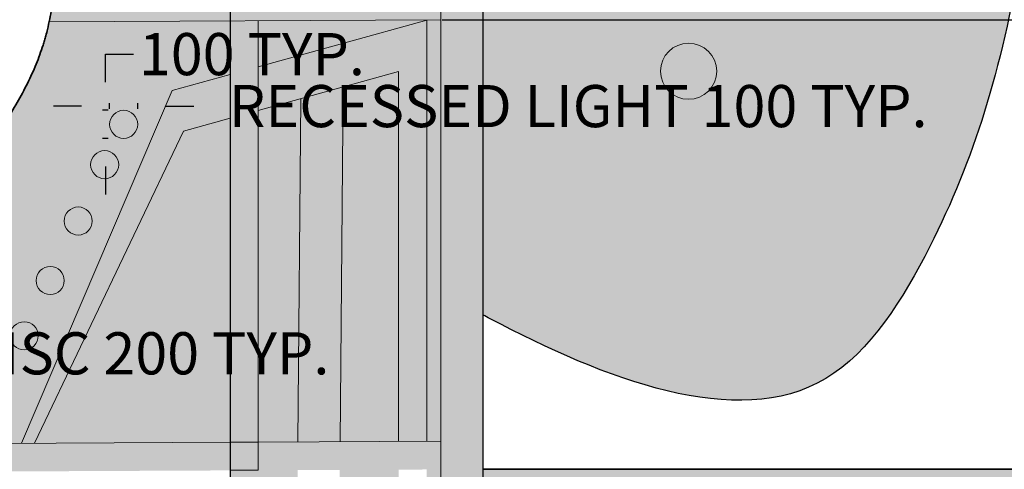
# Model space of a CAD drawing. Units: millimetres. Extents: x 11032 to 26788, y 3406 to 24505.
# Tile 69 of 78: x 21249 to 24753, y 11120 to 12721. Entities that reach past the tile are written whole.
import ezdxf

# ---------------------------------------------------------------- set-up
doc = ezdxf.new("R2010")
doc.units = ezdxf.units.MM
doc.header["$MEASUREMENT"] = 0
for name, color, linetype, lineweight in [('A-ANNO-DIMS', 2, 'Continuous', 18), ('A-GLAZ', 250, 'Continuous', 20), ('A-GLAZ-PATT', 9, 'Continuous', 13), ('A-ROOF', 7, 'Continuous', 30), ('A-WALL', 7, 'Continuous', 35), ('E-LITE', 7, 'Continuous', 18), ('E-LITE-PATT', 7, 'Continuous', 13)]:
    doc.layers.add(name, color=color, linetype=linetype, lineweight=lineweight)
for name, color, linetype, lineweight, true_color in [('A-GLAZ-FRAM-PATT', 250, 'Continuous', 13, 0x262627), ('A-ROOF-PATT', 9, 'Continuous', 13, 0xc7c8ca), ('A-WALL-CLAD-PATT', 9, 'Continuous', 13, 0xc7c8ca)]:
    doc.layers.add(name, color=color, linetype=linetype, lineweight=lineweight, true_color=true_color)
doc.styles.get("Standard").update_dxf_attribs({"font": 'arial.ttf'})
doc.dimstyles.get("Standard").update_dxf_attribs({"dimtxt": 150, "dimasz": 100, "dimexe": 10, "dimexo": 5, "dimgap": 5, "dimtad": 0, "dimtih": 1, "dimtoh": 1, "dimdec": 0, "dimzin": 0, "dimdsep": 46, "dimtxsty": 'Standard', "dimcen": 0.09, "dimadec": 0, "dimazin": 0, "dimtfac": 1, "dimtdec": 0, "dimtofl": 0, "dimtmove": 0, "dimatfit": 3, "dimfxl": 1, "dimtolj": 1, "dimtzin": 0, "dimarcsym": 0})

# ---------------------------------------------------------------- blocks, each defined once
blk = doc.blocks.new('RECESSED-LIGHT-100')
blk.add_circle((50, 50), 50)
blk = doc.blocks.new('RECESSED-LIGHT-200')
blk.add_circle((100, 100), 100)
blk = doc.blocks.new('*D20')
at = {"layer": 'A-ANNO-DIMS', "color": 0, "lineweight": -2, "transparency": 16777216}
for p, q in [((21468.9, 12413.4), (21368.9, 12413.4)), ((21568.9, 12403.4), (21568.9, 12423.4)), ((21668.9, 12403.4), (21668.9, 12423.4)), ((21768.9, 12413.4), (21868.9, 12413.4))]:
    blk.add_line(p, q, dxfattribs=at)
at = {"layer": 'A-ANNO-DIMS', "color": 0, "transparency": 16777216}
for points in [[(21468.9, 12430), (21468.9, 12396.7), (21568.9, 12413.4)], [(21768.9, 12430), (21768.9, 12396.7), (21668.9, 12413.4)]]:
    blk.add_solid(points, dxfattribs=at)
at = {"layer": 'Defpoints', "color": 0, "transparency": 16777216}
for p in [(21668.9, 12413.4), (21568.9, 12398.4), (21668.9, 12398.4)]:
    blk.add_point(p, dxfattribs=at)
at = {"layer": 'A-ANNO-DIMS', "color": 0, "transparency": 16777216, "insert": (23236.5, 12413.4), "char_height": 150, "attachment_point": 5}
blk.add_mtext('\\A1;RECESSED LIGHT 100 TYP.', dxfattribs=at)
blk = doc.blocks.new('*D21')
at = {"layer": 'A-ANNO-DIMS', "color": 0, "lineweight": -2, "transparency": 16777216}
for p, q in [((21553.9, 12498.4), (21553.9, 12598.4)), ((21553.9, 12598.4), (21653.9, 12598.4)), ((21563.9, 12398.4), (21543.9, 12398.4)), ((21563.9, 12298.4), (21543.9, 12298.4)), ((21553.9, 12198.4), (21553.9, 12098.4))]:
    blk.add_line(p, q, dxfattribs=at)
at = {"layer": 'A-ANNO-DIMS', "color": 0, "transparency": 16777216}
for points in [[(21537.2, 12498.4), (21570.6, 12498.4), (21553.9, 12398.4)], [(21537.2, 12198.4), (21570.6, 12198.4), (21553.9, 12298.4)]]:
    blk.add_solid(points, dxfattribs=at)
at = {"layer": 'Defpoints', "color": 0, "transparency": 16777216}
for p in [(21553.9, 12398.4), (21568.9, 12398.4), (21568.9, 12298.4)]:
    blk.add_point(p, dxfattribs=at)
at = {"layer": 'A-ANNO-DIMS', "color": 0, "transparency": 16777216, "insert": (22075.2, 12598.4), "char_height": 150, "attachment_point": 5}
blk.add_mtext('\\A1;100 TYP.', dxfattribs=at)
blk = doc.blocks.new('*D32')
at = {"layer": 'A-ANNO-DIMS', "color": 0, "lineweight": -2, "transparency": 16777216}
for p, q in [((19866, 11533.3), (19766, 11533.3)), ((19966, 11558.3), (19966, 11523.3)), ((20166, 11558.3), (20166, 11523.3)), ((20266, 11533.3), (20366, 11533.3))]:
    blk.add_line(p, q, dxfattribs=at)
at = {"layer": 'A-ANNO-DIMS', "color": 0, "transparency": 16777216}
for points in [[(19866, 11549.9), (19866, 11516.6), (19966, 11533.3)], [(20266, 11549.9), (20266, 11516.6), (20166, 11533.3)]]:
    blk.add_solid(points, dxfattribs=at)
at = {"layer": 'Defpoints', "color": 0, "transparency": 16777216}
for p in [(19966, 11563.3), (20166, 11563.3), (20166, 11533.3)]:
    blk.add_point(p, dxfattribs=at)
at = {"layer": 'A-ANNO-DIMS', "color": 0, "transparency": 16777216, "insert": (21400.3, 11533.3), "char_height": 150, "attachment_point": 5}
blk.add_mtext('\\A1;INLAY DISC 200 TYP.', dxfattribs=at)
blk = doc.blocks.new('*D36')
at = {"layer": 'A-ANNO-DIMS', "color": 0, "lineweight": -2, "transparency": 16777216}
for p, q in [((12301.3, 17115.9), (12301.3, 24416.9)), ((12401.3, 24406.9), (18569.2, 24406.9)), ((25297.4, 24406.9), (19129.5, 24406.9)), ((25397.4, 4466.4), (25397.4, 24416.9))]:
    blk.add_line(p, q, dxfattribs=at)
at = {"layer": 'A-ANNO-DIMS', "color": 0, "transparency": 16777216}
for points in [[(12401.3, 24423.5), (12401.3, 24390.2), (12301.3, 24406.9)], [(25297.4, 24423.5), (25297.4, 24390.2), (25397.4, 24406.9)]]:
    blk.add_solid(points, dxfattribs=at)
at = {"layer": 'Defpoints', "color": 0, "transparency": 16777216}
for p in [(25397.4, 24406.9), (12301.3, 17110.9), (25397.4, 4461.4)]:
    blk.add_point(p, dxfattribs=at)
at = {"layer": 'A-ANNO-DIMS', "color": 0, "transparency": 16777216, "insert": (18849.3, 24406.9), "char_height": 150, "attachment_point": 5}
blk.add_mtext('\\A1;13096', dxfattribs=at)
blk = doc.blocks.new('*D41')
at = {"layer": 'A-ANNO-DIMS', "color": 0, "lineweight": -2, "transparency": 16777216}
for p, q in [((22752.4, 12720.1), (26363.9, 12720.1)), ((26353.9, 12620.1), (26353.9, 12002)), ((26353.9, 11220.8), (26353.9, 11838.8)), ((25402.4, 11120.8), (26363.9, 11120.8))]:
    blk.add_line(p, q, dxfattribs=at)
at = {"layer": 'A-ANNO-DIMS', "color": 0, "transparency": 16777216}
for points in [[(26337.2, 12620.1), (26370.6, 12620.1), (26353.9, 12720.1)], [(26337.2, 11220.8), (26370.6, 11220.8), (26353.9, 11120.8)]]:
    blk.add_solid(points, dxfattribs=at)
at = {"layer": 'Defpoints', "color": 0, "transparency": 16777216}
for p in [(22747.4, 12720.1), (26353.9, 12720.1), (25397.4, 11120.8)]:
    blk.add_point(p, dxfattribs=at)
at = {"layer": 'A-ANNO-DIMS', "color": 0, "transparency": 16777216, "insert": (26353.9, 11920.4), "char_height": 150, "attachment_point": 5}
blk.add_mtext('\\A1;1599.3', dxfattribs=at)
blk = doc.blocks.new('*D42')
at = {"layer": 'A-ANNO-DIMS', "color": 0, "lineweight": -2, "transparency": 16777216}
for p, q in [((22752.4, 13320.1), (26363.9, 13320.1)), ((26353.9, 13220.1), (26353.9, 13101.7)), ((26353.9, 12820.1), (26353.9, 12938.5)), ((22752.4, 12720.1), (26363.9, 12720.1))]:
    blk.add_line(p, q, dxfattribs=at)
at = {"layer": 'A-ANNO-DIMS', "color": 0, "transparency": 16777216}
for points in [[(26337.2, 13220.1), (26370.6, 13220.1), (26353.9, 13320.1)], [(26337.2, 12820.1), (26370.6, 12820.1), (26353.9, 12720.1)]]:
    blk.add_solid(points, dxfattribs=at)
at = {"layer": 'Defpoints', "color": 0, "transparency": 16777216}
for p in [(22747.4, 13320.1), (26353.9, 13320.1), (22747.4, 12720.1)]:
    blk.add_point(p, dxfattribs=at)
at = {"layer": 'A-ANNO-DIMS', "color": 0, "transparency": 16777216, "insert": (26353.9, 13020.1), "char_height": 150, "attachment_point": 5}
blk.add_mtext('\\A1;600', dxfattribs=at)
blk = doc.blocks.new('*D51')
at = {"layer": 'A-ANNO-DIMS', "color": 0, "lineweight": -2, "transparency": 16777216}
for p, q in [((19697.4, 16000.7), (19697.4, 3494.9)), ((21997.4, 16011.6), (21997.4, 3494.9)), ((19797.4, 3504.9), (20617.4, 3504.9)), ((21897.4, 3504.9), (21077.4, 3504.9))]:
    blk.add_line(p, q, dxfattribs=at)
at = {"layer": 'A-ANNO-DIMS', "color": 0, "transparency": 16777216}
for points in [[(19797.4, 3521.6), (19797.4, 3488.2), (19697.4, 3504.9)], [(21897.4, 3521.6), (21897.4, 3488.2), (21997.4, 3504.9)]]:
    blk.add_solid(points, dxfattribs=at)
at = {"layer": 'Defpoints', "color": 0, "transparency": 16777216}
for p in [(21997.4, 16016.6), (19697.4, 16005.7), (21997.4, 3504.9)]:
    blk.add_point(p, dxfattribs=at)
at = {"layer": 'A-ANNO-DIMS', "color": 0, "transparency": 16777216, "insert": (20847.4, 3504.9), "char_height": 150, "attachment_point": 5}
blk.add_mtext('\\A1;2300', dxfattribs=at)
blk = doc.blocks.new('*D52')
at = {"layer": 'A-ANNO-DIMS', "color": 0, "lineweight": -2, "transparency": 16777216}
for p, q in [((22897.4, 16213.4), (22897.4, 3494.9)), ((21997.4, 16011.6), (21997.4, 3494.9)), ((22097.4, 3504.9), (22277, 3504.9)), ((22797.4, 3504.9), (22617.9, 3504.9))]:
    blk.add_line(p, q, dxfattribs=at)
at = {"layer": 'A-ANNO-DIMS', "color": 0, "transparency": 16777216}
for points in [[(22097.4, 3521.6), (22097.4, 3488.2), (21997.4, 3504.9)], [(22797.4, 3521.6), (22797.4, 3488.2), (22897.4, 3504.9)]]:
    blk.add_solid(points, dxfattribs=at)
at = {"layer": 'Defpoints', "color": 0, "transparency": 16777216}
for p in [(22897.4, 16218.4), (21997.4, 16016.6), (22897.4, 3504.9)]:
    blk.add_point(p, dxfattribs=at)
at = {"layer": 'A-ANNO-DIMS', "color": 0, "transparency": 16777216, "insert": (22447.4, 3504.9), "char_height": 150, "attachment_point": 5}
blk.add_mtext('\\A1;900', dxfattribs=at)
blk = doc.blocks.new('*D53')
at = {"layer": 'A-ANNO-DIMS', "color": 0, "lineweight": -2, "transparency": 16777216}
for p, q in [((22897.4, 11115.8), (22897.4, 3494.9)), ((25397.4, 11115.8), (25397.4, 3494.9)), ((22997.4, 3504.9), (23917.4, 3504.9)), ((25297.4, 3504.9), (24377.4, 3504.9))]:
    blk.add_line(p, q, dxfattribs=at)
at = {"layer": 'A-ANNO-DIMS', "color": 0, "transparency": 16777216}
for points in [[(22997.4, 3521.6), (22997.4, 3488.2), (22897.4, 3504.9)], [(25297.4, 3521.6), (25297.4, 3488.2), (25397.4, 3504.9)]]:
    blk.add_solid(points, dxfattribs=at)
at = {"layer": 'Defpoints', "color": 0, "transparency": 16777216}
for p in [(22897.4, 11120.8), (25397.4, 11120.8), (25397.4, 3504.9)]:
    blk.add_point(p, dxfattribs=at)
at = {"layer": 'A-ANNO-DIMS', "color": 0, "transparency": 16777216, "insert": (24147.4, 3504.9), "char_height": 150, "attachment_point": 5}
blk.add_mtext('\\A1;2500', dxfattribs=at)

msp = doc.modelspace()

# ---------------------------------------------------------------- hatches: boundary and pattern name
at = {"layer": 'A-GLAZ-FRAM-PATT'}
h = msp.add_hatch(color=256, dxfattribs=at)
h.paths.add_polyline_path([(22747.404, 16218.44), (22395.025, 16218.44), (18518.2, 16200.148), (18519.143, 16000.151), (22747.404, 16020.1)])
edge = h.paths.add_edge_path()
edge.add_line((22897.404, 16218.44), (22747.404, 16218.44))
edge.add_line((22747.404, 16218.44), (22747.404, 16020.1))
edge.add_line((22747.404, 16020.1), (22747.404, 9631.346))
edge.add_spline(control_points=[(22747.404, 9631.346), (22803.273, 9520.228), (22853.467, 9405.87), (22897.404, 9289.211)], knot_values=[2645.78092422, 2645.78092422, 2645.78092422, 2645.78092422, 3013.05623672, 3013.05623672, 3013.05623672, 3013.05623672], degree=3, periodic=0)
edge.add_line((22897.404, 9289.211), (22897.404, 16218.44))
h.paths.add_polyline_path([(22097.404, 16017.033), (21997.404, 16016.562), (21997.404, 13316.532), (22097.404, 13317.003)])
edge = h.paths.add_edge_path()
edge.add_line((19797.404, 16006.182), (19697.404, 16005.71))
edge.add_line((19697.404, 16005.71), (19697.404, 15155.703))
edge.add_line((19697.404, 15155.703), (19697.404, 12747.012))
edge.add_spline(control_points=[(19697.404, 12747.012), (19708.389, 12750.081), (19719.253, 12753.406), (19732.457, 12757.789), (19734.918, 12758.62), (19737.372, 12759.464)], knot_values=[1372.60477099, 1372.60477099, 1372.60477099, 1372.60477099, 1399.44343377, 1399.44343377, 1405.61279972, 1405.61279972, 1405.61279972, 1405.61279972], degree=3, periodic=0)
edge.add_spline(control_points=[(19737.372, 12759.464), (19750.245, 12763.891), (19762.932, 12768.657), (19778.9, 12775.14), (19782.354, 12776.572), (19785.794, 12778.028)], knot_values=[1405.61279972, 1405.61279972, 1405.61279972, 1405.61279972, 1437.96891336, 1437.96891336, 1446.94640473, 1446.94640473, 1446.94640473, 1446.94640473], degree=3, periodic=0)
edge.add_spline(control_points=[(19785.794, 12778.028), (19789.682, 12779.673), (19793.552, 12781.348), (19797.404, 12783.051)], knot_values=[1446.94640473, 1446.94640473, 1446.94640473, 1446.94640473, 1457.09545574, 1457.09545574, 1457.09545574, 1457.09545574], degree=3, periodic=0)
edge.add_line((19797.404, 12783.051), (19797.404, 15306.174))
edge.add_line((19797.404, 15306.174), (19797.404, 16006.182))
h = msp.add_hatch(color=256, dxfattribs=at)
h.paths.add_polyline_path([(22747.404, 16020.1), (22697.404, 16019.864), (22697.404, 15169.858), (22747.404, 15170.094)])
h.paths.add_polyline_path([(22747.404, 15070.092), (22697.404, 15069.857), (22697.404, 13319.834), (22747.404, 13320.07)])
edge = h.paths.add_edge_path()
edge.add_line((22747.404, 12795.064), (21365.955, 12788.546))
edge.add_spline(control_points=[(21365.955, 12788.546), (21365.556, 12785.216), (21365.14, 12781.894), (21364.707, 12778.582)], knot_values=[4871.89074498, 4871.89074498, 4871.89074498, 4871.89074498, 4881.51384723, 4881.51384723, 4881.51384723, 4881.51384723], degree=3, periodic=0)
edge.add_spline(control_points=[(21364.707, 12778.582), (21363.953, 12772.805), (21363.147, 12767.057), (21359.867, 12745.141), (21357.035, 12729.186), (21353.796, 12713.488)], knot_values=[4881.51384723, 4881.51384723, 4881.51384723, 4881.51384723, 4898.30109774, 4898.30109774, 4945.85686537, 4945.85686537, 4945.85686537, 4945.85686537], degree=3, periodic=0)
edge.add_line((21353.796, 12713.488), (22747.404, 12720.064))
edge.add_line((22747.404, 12720.064), (22747.404, 12795.064))
edge = h.paths.add_edge_path()
edge.add_line((22747.404, 13320.07), (22697.404, 13319.834))
edge.add_line((22697.404, 13319.834), (21312.567, 13313.3))
edge.add_spline(control_points=[(21312.567, 13313.3), (21312.567, 13313.3), (21312.567, 13313.3), (21312.567, 13313.3)], knot_values=[4405.86932069, 4405.86932069, 4405.86932069, 4405.86932069, 4405.86932536, 4405.86932536, 4405.86932536, 4405.86932536], degree=3, periodic=0)
edge.add_spline(control_points=[(21312.567, 13313.3), (21316.329, 13300.292), (21319.935, 13287.252), (21326.522, 13262.273), (21329.53, 13250.337), (21332.397, 13238.393)], knot_values=[4405.86932536, 4405.86932536, 4405.86932536, 4405.86932536, 4439.73791994, 4439.73791994, 4470.65028407, 4470.65028407, 4470.65028407, 4470.65028407], degree=3, periodic=0)
edge.add_line((21332.397, 13238.393), (22747.404, 13245.069))
edge.add_line((22747.404, 13245.069), (22747.404, 13320.07))
h.paths.add_polyline_path([(22747.404, 13245.069), (22697.404, 13244.833), (22697.404, 12794.828), (22747.404, 12795.064)])
h.paths.add_polyline_path([(22747.404, 12720.064), (22697.404, 12719.828), (22697.404, 11219.811), (22747.404, 11220.047)])
edge = h.paths.add_edge_path()
edge.add_line((22747.404, 11120.046), (22697.404, 11119.81))
edge.add_line((22697.404, 11119.81), (22697.404, 9727.135))
edge.add_spline(control_points=[(22697.404, 9727.135), (22714.538, 9695.493), (22731.209, 9663.555), (22747.404, 9631.346)], knot_values=[2539.32128955, 2539.32128955, 2539.32128955, 2539.32128955, 2645.78092422, 2645.78092422, 2645.78092422, 2645.78092422], degree=3, periodic=0)
edge.add_line((22747.404, 9631.346), (22747.404, 11120.046))
h = msp.add_hatch(color=256, dxfattribs=at)
h.paths.add_polyline_path([(21997.404, 12525.979), (21791.467, 12468.949), (21255.866, 11213.01), (21301.184, 11213.223), (21831.499, 12324.39), (21997.404, 12370.333)])
h.paths.add_polyline_path([(22697.404, 12719.828), (22097.404, 12716.997), (22097.404, 12553.671)])
h = msp.add_hatch(color=256, dxfattribs=at)
h.paths.add_polyline_path([(22097.404, 12716.997), (21997.404, 12716.525), (21997.404, 11216.508), (22097.404, 11216.508)])
h.paths.add_polyline_path([(22747.404, 11220.047), (22097.404, 11216.98), (22097.404, 11116.979), (22747.404, 11120.046)])
edge = h.paths.add_edge_path()
edge.add_line((22097.404, 11116.979), (21997.404, 11116.979))
edge.add_line((21997.404, 11116.979), (21997.404, 10579.29))
edge.add_spline(control_points=[(21997.404, 10579.29), (22031.89, 10555.567), (22065.161, 10529.697), (22097.404, 10502.28)], knot_values=[1427.45738773, 1427.45738773, 1427.45738773, 1427.45738773, 1555.90366196, 1555.90366196, 1555.90366196, 1555.90366196], degree=3, periodic=0)
edge.add_line((22097.404, 10502.28), (22097.404, 11116.979))
h.paths.add_polyline_path([(22097.404, 11216.508), (21997.404, 11216.508), (21997.404, 11116.979), (22097.404, 11116.979)])
h = msp.add_hatch(color=256, dxfattribs=at)
edge = h.paths.add_edge_path()
edge.add_line((21997.404, 11116.507), (21997.404, 11216.508))
edge.add_line((21997.404, 11216.508), (20604.964, 11209.938))
edge.add_spline(control_points=[(20604.964, 11209.938), (20607.134, 11206.535), (20609.342, 11203.201), (20617.481, 11191.329), (20623.597, 11183.201), (20636.089, 11167.852), (20642.464, 11160.629), (20655.347, 11147.002), (20661.856, 11140.596), (20674.924, 11128.498), (20681.484, 11122.806), (20690.98, 11115.01), (20693.915, 11112.662), (20696.848, 11110.371)], knot_values=[6471.16279551, 6471.16279551, 6471.16279551, 6471.16279551, 6478.49642841, 6478.49642841, 6497.82694928, 6497.82694928, 6517.15747016, 6517.15747016, 6536.48799103, 6536.48799103, 6555.81851191, 6555.81851191, 6564.46246221, 6564.46246221, 6564.46246221, 6564.46246221], degree=3, periodic=0)
edge.add_line((20696.848, 11110.371), (21997.404, 11116.507))
at = {"layer": 'A-GLAZ-PATT'}
h = msp.add_hatch(color=256, dxfattribs=at)
h.set_gradient(color1=(147, 149, 152), color2=(254, 234, 185), name='INVCURVED')
h.paths.add_polyline_path([(22597.404, 11219.339), (22697.404, 11219.811), (22697.404, 12719.828), (22097.404, 12553.671), (22097.404, 12398.026), (22597.404, 12536.49)])
h.paths.add_polyline_path([(22399.472, 12481.677), (22249.118, 12440.04), (22238.879, 11217.648), (22388.89, 11218.355)])
h = msp.add_hatch(color=256, dxfattribs=at)
h.set_gradient(color1=(254, 204, 102), color2=(248, 246, 176), name='HEMISPHERICAL')
edge = h.paths.add_edge_path()
edge.add_spline(control_points=[(21353.796, 12713.488), (21351.921, 12704.4), (21349.909, 12695.398), (21345.944, 12678.95), (21344.029, 12671.478), (21341.252, 12661.256), (21340.473, 12658.452), (21338.881, 12652.839), (21338.068, 12650.032), (21335.58, 12641.609), (21333.854, 12635.993), (21328.479, 12619.14), (21324.632, 12607.899), (21312.219, 12573.877), (21302.855, 12551.077), (21282.165, 12505.474), (21270.839, 12482.672), (21246.416, 12437.152), (21233.319, 12414.435), (21205.588, 12369.182), (21190.953, 12346.647), (21160.407, 12301.852), (21144.496, 12279.592), (21111.679, 12235.428), (21094.773, 12213.524), (21055.718, 12164.423), (21033.359, 12137.352), (20988.115, 12083.954), (20965.231, 12057.628), (20919.516, 12005.731), (20896.686, 11980.16), (20857.367, 11936.124), (20840.745, 11917.509), (20808.035, 11880.563), (20791.947, 11862.233), (20763.475, 11829.178), (20750.967, 11814.43), (20726.5, 11784.882), (20714.539, 11770.084), (20693.385, 11742.981), (20684.087, 11730.721), (20665.941, 11705.856), (20657.092, 11693.252), (20641.315, 11669.592), (20634.312, 11658.625), (20620.703, 11636.087), (20614.097, 11624.517), (20601.376, 11600.52), (20595.259, 11588.093), (20585.03, 11565.079), (20580.781, 11554.73), (20572.815, 11533.181), (20569.097, 11521.98), (20562.398, 11498.577), (20559.418, 11486.373), (20555.045, 11463.74), (20553.448, 11453.531), (20551.046, 11432.459), (20550.243, 11421.596), (20549.62, 11399.291), (20549.802, 11387.848), (20551.33, 11364.54), (20552.678, 11352.676), (20556.671, 11328.775), (20559.317, 11316.74), (20565.954, 11292.813), (20569.944, 11280.922), (20579.202, 11257.616), (20584.469, 11246.202), (20592.114, 11231.712), (20593.991, 11228.293), (20597.158, 11222.745), (20598.418, 11220.59), (20600.975, 11216.322), (20602.269, 11214.214), (20604.037, 11211.397), (20604.5, 11210.666), (20604.964, 11209.938)], knot_values=[4945.85686537, 4945.85686537, 4945.85686537, 4945.85686537, 4973.3893459, 4973.3893459, 4996.66899489, 4996.66899489, 5005.51338613, 5005.51338613, 5014.35777737, 5014.35777737, 5032.04655985, 5032.04655985, 5067.42412481, 5067.42412481, 5139.05868364, 5139.05868364, 5210.69324248, 5210.69324248, 5282.32780131, 5282.32780131, 5353.96236015, 5353.96236015, 5425.59691898, 5425.59691898, 5497.23147782, 5497.23147782, 5587.7210555, 5587.7210555, 5678.21063318, 5678.21063318, 5768.70021086, 5768.70021086, 5836.11850381, 5836.11850381, 5903.53679676, 5903.53679676, 5958.13178915, 5958.13178915, 6012.72678154, 6012.72678154, 6057.24703228, 6057.24703228, 6101.76728303, 6101.76728303, 6138.92040589, 6138.92040589, 6176.07352875, 6176.07352875, 6213.2266516, 6213.2266516, 6241.78247951, 6241.78247951, 6270.33830742, 6270.33830742, 6298.89413533, 6298.89413533, 6321.01839771, 6321.01839771, 6343.1426601, 6343.1426601, 6365.26692248, 6365.26692248, 6387.39118486, 6387.39118486, 6409.51544725, 6409.51544725, 6431.63970963, 6431.63970963, 6453.76397201, 6453.76397201, 6460.69362746, 6460.69362746, 6465.1443277, 6465.1443277, 6469.59502793, 6469.59502793, 6471.16279551, 6471.16279551, 6471.16279551, 6471.16279551], degree=3, periodic=0)
edge.add_line((20604.964, 11209.938), (21255.866, 11213.01))
edge.add_line((21255.866, 11213.01), (21791.467, 12468.949))
edge.add_line((21791.467, 12468.949), (21997.404, 12525.979))
edge.add_line((21997.404, 12525.979), (21997.404, 12716.525))
edge.add_line((21997.404, 12716.525), (21353.796, 12713.488))
h.paths.add_polyline_path([(21407.506, 11792.395, -1), (21307.506, 11792.395, -1)], flags=16)
h.paths.add_polyline_path([(21315.053, 11595.746, -1), (21215.053, 11595.746, -1)], flags=16)
h.paths.add_polyline_path([(21407.11, 12004.255, -1), (21507.11, 12004.255, -1)], flags=16)
h.paths.add_polyline_path([(21220.849, 11395.371, -1), (21120.849, 11395.371, -1)], flags=16)
h.paths.add_polyline_path([(21501.367, 12204.741, -1), (21601.367, 12204.741, -1)], flags=16)
h.paths.add_polyline_path([(21568.897, 12348.379, -1), (21668.897, 12348.379, -1)], flags=16)
h = msp.add_hatch(color=256, dxfattribs=at)
h.set_gradient(color1=(254, 234, 185), color2=(247, 242, 129), name='SPHERICAL')
h.paths.add_polyline_path([(22097.404, 11216.98), (22238.879, 11217.648), (22249.118, 12440.04), (22097.404, 12398.026)])
h.paths.add_polyline_path([(22597.404, 12536.49), (22399.472, 12481.677), (22388.89, 11218.355), (22597.404, 11219.339)])
edge = h.paths.add_edge_path()
edge.add_spline(control_points=[(22380.418, 10206.878), (22458.962, 10109.885), (22531.093, 10007.052), (22597.404, 9899.872)], knot_values=[1967.32460229, 1967.32460229, 1967.32460229, 1967.32460229, 2342.00276579, 2342.00276579, 2342.00276579, 2342.00276579], degree=3, periodic=0)
edge.add_line((22597.404, 9899.872), (22597.404, 10880.68))
edge.add_line((22597.404, 10880.68), (22385.926, 10864.474))
edge.add_line((22385.926, 10864.474), (22380.418, 10206.878))
edge = h.paths.add_edge_path()
edge.add_spline(control_points=[(22097.404, 10502.28), (22137.084, 10468.539), (22182.031, 10425.998), (22225.292, 10381.762), (22231.821, 10375.007)], knot_values=[1555.90366196, 1555.90366196, 1555.90366196, 1555.90366196, 1713.9810301, 1742.27732176, 1742.27732176, 1742.27732176, 1742.27732176], degree=3, periodic=0)
edge.add_line((22231.821, 10375.007), (22238.042, 11117.642))
edge.add_line((22238.042, 11117.642), (22097.404, 11116.979))
edge.add_line((22097.404, 11116.979), (22097.404, 10502.28))
h.paths.add_polyline_path([(22597.404, 10980.973), (22597.404, 11119.338), (22388.053, 11118.35), (22386.767, 10964.831)])
h = msp.add_hatch(color=256, dxfattribs=at)
h.set_gradient(color1=(254, 204, 102), color2=(248, 246, 176), name='HEMISPHERICAL')
h.paths.add_polyline_path([(21997.404, 12370.333), (21831.499, 12324.39), (21301.184, 11213.223), (21997.404, 11216.508)])
at = {"layer": 'A-ROOF-PATT'}
h = msp.add_hatch(color=256, dxfattribs=at)
h.set_gradient(color1=(254, 234, 185), color2=(254, 204, 102), name='HEMISPHERICAL')
edge = h.paths.add_edge_path()
edge.add_spline(control_points=[(22897.404, 11669.966), (22905.925, 11665.421), (23315.936, 11448.075), (24040.798, 11159.928), (24591.756, 12047.169), (24823.737, 12810.982), (24947.403, 13888.961), (24865.187, 14241.353)], knot_values=[3287.74811127, 3287.74811127, 3287.74811127, 3287.74811127, 3313.95061448, 4543.69878516, 5160.49832431, 6201.61230094, 7164.26935092, 7164.26935092, 7164.26935092, 7164.26935092], degree=3, periodic=0)
edge.add_spline(control_points=[(24865.187, 14241.353), (24864.423, 14242.575), (24766.311, 14398.016), (24602.876, 14465.087), (24430.499, 14490.269)], knot_values=[2462.20964139, 2462.20964139, 2462.20964139, 2462.20964139, 2466.8266732, 3052.28296943, 3052.28296943, 3052.28296943, 3052.28296943], degree=3, periodic=0)
edge.add_spline(control_points=[(24430.499, 14490.269), (24425.883, 14491.82), (24421.191, 14493.323), (24402.038, 14499.174), (24386.985, 14503.129), (24351.089, 14511.181), (24329.855, 14514.969), (24285.944, 14521.074), (24263.27, 14523.392), (24216.998, 14526.696), (24193.401, 14527.682), (24156.534, 14528.34), (24143.408, 14528.404), (24117.112, 14528.234), (24103.938, 14528.001), (24070.613, 14527.088), (24050.758, 14526.245), (24021.415, 14524.553), (24011.706, 14523.918), (23966.994, 14520.648), (23932.846, 14517.154), (23866.075, 14508.38), (23833.453, 14503.099), (23769.399, 14490.798), (23737.967, 14483.778), (23675.954, 14468.02), (23645.373, 14459.282), (23584.735, 14440.092), (23554.677, 14429.638), (23494.779, 14407.002), (23464.938, 14394.819), (23420.13, 14375.236), (23405.186, 14368.49), (23382.735, 14358.043), (23375.245, 14354.506), (23363.999, 14349.118), (23360.248, 14347.308), (23354.645, 14344.586), (23352.794, 14343.684), (23350.017, 14342.326), (23349.099, 14341.876), (23346.705, 14340.7), (23345.24, 14339.978), (23338.743, 14336.765), (23333.903, 14334.336), (23322.952, 14328.714), (23316.906, 14325.517), (23304.544, 14318.72), (23298.224, 14315.118), (23284.755, 14307.106), (23277.606, 14302.694), (23262.032, 14292.682), (23253.61, 14287.081), (23235.154, 14274.351), (23225.122, 14267.224), (23200.911, 14249.486), (23186.304, 14238.46), (23150.266, 14210.435), (23128.041, 14192.649), (23080.227, 14153.32), (23055.083, 14132.223), (23027.357, 14108.523)], knot_values=[765.02120011, 765.02120011, 765.02120011, 765.02120011, 788.26421035, 788.26421035, 858.47024111, 858.47024111, 949.55129088, 949.55129088, 1040.63234064, 1040.63234064, 1131.71339041, 1131.71339041, 1181.69353236, 1181.69353236, 1231.67367431, 1231.67367431, 1308.31901537, 1308.31901537, 1346.64168591, 1346.64168591, 1486.09404767, 1486.09404767, 1625.54640943, 1625.54640943, 1764.99877119, 1764.99877119, 1904.45113295, 1904.45113295, 2043.90349471, 2043.90349471, 2183.35585648, 2183.35585648, 2253.08203736, 2253.08203736, 2287.9451278, 2287.9451278, 2305.37667302, 2305.37667302, 2313.97014819, 2313.97014819, 2318.26688578, 2318.26688578, 2325.26983634, 2325.26983634, 2349.68341829, 2349.68341829, 2381.60377634, 2381.60377634, 2413.52413439, 2413.52413439, 2445.44449243, 2445.44449243, 2477.36485048, 2477.36485048, 2509.28520853, 2509.28520853, 2547.80727814, 2547.80727814, 2595.07704725, 2595.07704725, 2638.35089074, 2638.35089074, 2638.35089074, 2638.35089074], degree=3, periodic=0)
edge.add_spline(control_points=[(23027.357, 14108.523), (23027.349, 14108.516), (23027.342, 14108.51), (23027.334, 14108.504), (22984.024, 14071.482), (22940.714, 14034.46), (22897.404, 13997.439)], knot_values=[697.41436256, 697.41436256, 697.41436256, 697.41436256, 697.4261083, 697.4261083, 697.4261083, 765.02120011, 765.02120011, 765.02120011, 765.02120011], degree=3, periodic=0)
edge.add_line((22897.404, 13997.439), (22897.404, 11669.966))
h.paths.add_polyline_path([(23729.349, 12537.488, -1), (23529.349, 12537.488, -1)], flags=16)
h.paths.add_polyline_path([(23963.611, 13699.89, -1), (24163.611, 13699.89, -1)], flags=16)
at = {"layer": 'A-WALL-CLAD-PATT'}
h = msp.add_hatch(color=256, dxfattribs=at)
edge = h.paths.add_edge_path()
edge.add_spline(control_points=[(24865.187, 14241.353), (24844.683, 14329.238), (24708.481, 14689.762), (23980.011, 14777.842), (23439.65, 14624.598), (23111.535, 14443.589), (22897.404, 14260.55)], knot_values=[765.02120011, 765.02120011, 765.02120011, 765.02120011, 1005.10337375, 1880.54593672, 2963.32805357, 3287.74811127, 3287.74811127, 3287.74811127, 3287.74811127], degree=3, periodic=0)
edge.add_line((22897.404, 14260.55), (22897.404, 13997.439))
edge.add_spline(control_points=[(22897.404, 13997.439), (22940.714, 14034.46), (22984.024, 14071.482), (23027.334, 14108.504), (23027.342, 14108.51), (23027.349, 14108.516), (23027.357, 14108.523)], knot_values=[697.41436256, 697.41436256, 697.41436256, 697.41436256, 765.00945437, 765.00945437, 765.00945437, 765.02120011, 765.02120011, 765.02120011, 765.02120011], degree=3, periodic=0)
edge.add_spline(control_points=[(23027.357, 14108.523), (23055.083, 14132.223), (23080.227, 14153.32), (23128.041, 14192.649), (23150.266, 14210.435), (23186.304, 14238.46), (23200.911, 14249.486), (23225.122, 14267.224), (23235.154, 14274.351), (23253.61, 14287.081), (23262.032, 14292.682), (23277.606, 14302.694), (23284.755, 14307.106), (23298.224, 14315.118), (23304.544, 14318.72), (23316.906, 14325.517), (23322.952, 14328.714), (23333.903, 14334.336), (23338.743, 14336.765), (23345.24, 14339.978), (23346.705, 14340.7), (23349.099, 14341.876), (23350.017, 14342.326), (23352.794, 14343.684), (23354.645, 14344.586), (23360.248, 14347.308), (23363.999, 14349.118), (23375.245, 14354.506), (23382.735, 14358.043), (23405.186, 14368.49), (23420.13, 14375.236), (23464.938, 14394.819), (23494.779, 14407.002), (23554.677, 14429.638), (23584.735, 14440.092), (23645.373, 14459.282), (23675.954, 14468.02), (23737.967, 14483.778), (23769.399, 14490.798), (23833.453, 14503.099), (23866.075, 14508.38), (23932.846, 14517.154), (23966.994, 14520.648), (24011.706, 14523.918), (24021.415, 14524.553), (24050.758, 14526.245), (24070.613, 14527.088), (24103.938, 14528.001), (24117.112, 14528.234), (24143.408, 14528.404), (24156.534, 14528.34), (24193.401, 14527.682), (24216.998, 14526.696), (24263.27, 14523.392), (24285.944, 14521.074), (24329.855, 14514.969), (24351.089, 14511.181), (24386.985, 14503.129), (24402.038, 14499.174), (24421.191, 14493.323), (24425.883, 14491.82), (24430.499, 14490.269)], knot_values=[765.02120011, 765.02120011, 765.02120011, 765.02120011, 808.29504361, 808.29504361, 855.56481272, 855.56481272, 894.08688233, 894.08688233, 926.00724037, 926.00724037, 957.92759842, 957.92759842, 989.84795647, 989.84795647, 1021.76831451, 1021.76831451, 1053.68867256, 1053.68867256, 1078.10225451, 1078.10225451, 1085.10520508, 1085.10520508, 1089.40194266, 1089.40194266, 1097.99541784, 1097.99541784, 1115.42696306, 1115.42696306, 1150.2900535, 1150.2900535, 1220.01623438, 1220.01623438, 1359.46859614, 1359.46859614, 1498.9209579, 1498.9209579, 1638.37331966, 1638.37331966, 1777.82568142, 1777.82568142, 1917.27804319, 1917.27804319, 2056.73040495, 2056.73040495, 2095.05307548, 2095.05307548, 2171.69841654, 2171.69841654, 2221.67855849, 2221.67855849, 2271.65870045, 2271.65870045, 2362.73975021, 2362.73975021, 2453.82079998, 2453.82079998, 2544.90184974, 2544.90184974, 2615.10788051, 2615.10788051, 2638.35089074, 2638.35089074, 2638.35089074, 2638.35089074], degree=3, periodic=0)
edge.add_spline(control_points=[(24430.499, 14490.269), (24602.876, 14465.087), (24766.311, 14398.016), (24864.423, 14242.575), (24865.187, 14241.353)], knot_values=[2462.20964139, 2462.20964139, 2462.20964139, 2462.20964139, 3047.66593763, 3052.28296943, 3052.28296943, 3052.28296943, 3052.28296943], degree=3, periodic=0)
h.paths.add_polyline_path([(25397.404, 11120.753), (22897.404, 11120.753), (22897.404, 10520.753), (25197.404, 10520.753), (25197.404, 9359.601), (25397.404, 9359.601)])
at = {"layer": 'E-LITE-PATT'}
h = msp.add_hatch(color=256, dxfattribs=at)
h.paths.add_polyline_path([(23729.349, 12537.488, 1), (23529.349, 12537.488, 1)])
h.paths.add_polyline_path([(24163.611, 13699.89, 1), (23963.611, 13699.89, 1)])
h.paths.add_polyline_path([(18790.086, 14298.34, 1), (18890.086, 14298.34, 1)])
h.paths.add_polyline_path([(19537.524, 14550.125, 1), (19437.524, 14550.125, 1)])
h.paths.add_polyline_path([(20194.664, 14380.821, 1), (20344.664, 14380.821, 1)])
h.paths.add_polyline_path([(20018.772, 14780.204, 1), (19868.772, 14780.204, 1)])
h.paths.add_polyline_path([(20594.425, 14224.541, 1), (20744.425, 14224.541, 1)])
h.paths.add_polyline_path([(21232.101, 14202.835, 1), (21332.101, 14202.835, 1)])
h.paths.add_polyline_path([(20854.127, 14602.218, 1), (20754.127, 14602.218, 1)])
h.paths.add_polyline_path([(21492.875, 14667.335, 1), (21392.875, 14667.335, 1)])
h.paths.add_polyline_path([(21005.138, 14988.578, 1), (20855.138, 14988.578, 1)])
h = msp.add_hatch(color=256, dxfattribs=at)
h.paths.add_polyline_path([(21120.849, 11395.371, 1), (21220.849, 11395.371, 1)])
h.paths.add_polyline_path([(21215.053, 11595.746, 1), (21315.053, 11595.746, 1)])
h.paths.add_polyline_path([(21407.506, 11792.395, 1), (21307.506, 11792.395, 1)])
h.paths.add_polyline_path([(21507.11, 12004.255, 1), (21407.11, 12004.255, 1)])
h.paths.add_polyline_path([(21501.367, 12204.741, 1), (21601.367, 12204.741, 1)])
h.paths.add_polyline_path([(21668.897, 12348.379, 1), (21568.897, 12348.379, 1)])
h.paths.add_polyline_path([(23729.349, 12537.488, 1), (23529.349, 12537.488, 1)])
h.paths.add_polyline_path([(23963.611, 13699.89, 1), (24163.611, 13699.89, 1)])
h.paths.add_polyline_path([(21492.875, 14667.335, 1), (21392.875, 14667.335, 1)])
h.paths.add_polyline_path([(21332.101, 14202.835, 1), (21232.101, 14202.835, 1)])
h.paths.add_polyline_path([(20744.425, 14224.541, 1), (20594.425, 14224.541, 1)])
h.paths.add_polyline_path([(20854.127, 14602.218, 1), (20754.127, 14602.218, 1)])
h.paths.add_polyline_path([(20947.253, 15061.599), (20912.335, 15061.434, 0.34563694), (20855.138, 14988.578, 1), (21005.138, 14988.578, 0.34827999)])
h = msp.add_hatch(color=256, dxfattribs=at)
h.paths.add_polyline_path([(23529.349, 12537.488, 1), (23729.349, 12537.488, 1)])
h.paths.add_polyline_path([(24163.611, 13699.89, 1), (23963.611, 13699.89, 1)])

# ---------------------------------------------------------------- linework, layer by layer
at = {"layer": 'A-GLAZ'}
for p, q in [((22747.404, 16218.44), (22747.404, 9631.346)), ((22897.404, 16218.44), (22897.404, 9289.211)), ((22747.404, 12720.064), (21353.796, 12713.488)), ((22697.404, 12719.828), (22097.404, 12553.671)), ((22697.404, 12719.828), (22697.404, 11219.811)), ((21997.404, 12716.525), (21997.404, 11216.508)), ((22097.404, 12716.997), (22097.404, 11216.98)), ((21997.404, 12525.979), (21791.467, 12468.949)), ((22597.404, 12536.49), (22097.404, 12398.026)), ((22597.404, 12536.49), (22597.404, 11219.811)), ((22399.472, 12481.677), (22388.89, 11218.355)), ((21791.467, 12468.949), (21255.866, 11213.01)), ((22249.118, 12440.04), (22238.879, 11217.648)), ((21997.404, 12370.333), (21831.499, 12324.39)), ((21831.499, 12324.39), (21301.184, 11213.223)), ((21997.404, 11216.508), (20604.964, 11209.938)), ((22747.404, 11220.047), (22097.404, 11216.98))]:
    msp.add_line(p, q, dxfattribs=at)
msp.add_lwpolyline([(21997.404, 11216.508), (22097.404, 11216.508), (22097.404, 11116.979), (21997.404, 11116.979)], close=True, dxfattribs=at)
at = {"layer": 'A-ROOF'}
msp.add_open_spline([(22897.404, 14260.55), (23111.535, 14443.589), (23439.65, 14624.598), (23980.011, 14777.842), (25027.484, 14651.191), (24844.989, 12880.959), (24591.756, 12047.169), (24040.798, 11159.928), (23315.936, 11448.075), (22905.925, 11665.421), (22897.404, 11669.966)], degree=3, knots=[765.02120011, 765.02120011, 765.02120011, 765.02120011, 1089.44125781, 2172.22337467, 3047.66593763, 4250.40516126, 5291.51913789, 5908.31867703, 7138.06684772, 7164.26935092, 7164.26935092, 7164.26935092, 7164.26935092], dxfattribs=at)
at = {"layer": 'A-WALL'}
msp.add_line((22897.404, 11120.753), (25397.404, 11120.753), dxfattribs=at)
msp.add_open_spline([(20781.73, 14097.965), (20784.285, 14097.292), (20787.436, 14096.331), (20794.831, 14093.655), (20799.074, 14091.941), (20808.517, 14087.64), (20813.716, 14085.055), (20824.925, 14078.948), (20830.934, 14075.426), (20843.621, 14067.418), (20850.299, 14062.932), (20864.197, 14052.997), (20871.416, 14047.547), (20889.597, 14033.059), (20900.79, 14023.505), (20923.774, 14002.511), (20935.566, 13991.072), (20959.505, 13966.429), (20971.653, 13953.226), (20996.104, 13925.188), (21008.407, 13910.354), (21032.993, 13879.192), (21045.278, 13862.864), (21075.715, 13820.438), (21093.762, 13793.504), (21129.039, 13737.067), (21146.269, 13707.566), (21179.532, 13646.451), (21195.565, 13614.838), (21226.093, 13549.956), (21240.587, 13516.686), (21267.729, 13448.943), (21280.375, 13414.47), (21303.538, 13344.776), (21314.054, 13309.556), (21332.704, 13238.828), (21340.837, 13203.321), (21354.5, 13132.481), (21360.029, 13097.149), (21368.306, 13027.119), (21371.052, 12992.421), (21373.63, 12924.101), (21373.462, 12890.481), (21370.13, 12824.718), (21366.968, 12792.577), (21358.463, 12735.763), (21353.621, 12710.793), (21345.944, 12678.95), (21344.029, 12671.478), (21341.252, 12661.256), (21340.473, 12658.452), (21338.881, 12652.839), (21338.068, 12650.032), (21335.58, 12641.609), (21333.854, 12635.993), (21328.479, 12619.14), (21324.632, 12607.899), (21312.219, 12573.877), (21302.855, 12551.077), (21282.165, 12505.474), (21270.839, 12482.672), (21246.416, 12437.152), (21233.319, 12414.435), (21205.588, 12369.182), (21190.953, 12346.647), (21160.407, 12301.852), (21144.496, 12279.592), (21111.679, 12235.428), (21094.773, 12213.524), (21055.718, 12164.423), (21033.359, 12137.352), (20988.115, 12083.954), (20965.231, 12057.628), (20919.516, 12005.731), (20896.686, 11980.16), (20857.367, 11936.124), (20840.745, 11917.509), (20808.035, 11880.563), (20791.947, 11862.233), (20763.475, 11829.178), (20750.967, 11814.43), (20726.5, 11784.882), (20714.539, 11770.084), (20693.385, 11742.981), (20684.087, 11730.721), (20665.941, 11705.856), (20657.092, 11693.252), (20641.315, 11669.592), (20634.312, 11658.625), (20620.703, 11636.087), (20614.097, 11624.517), (20601.376, 11600.52), (20595.259, 11588.093), (20585.03, 11565.079), (20580.781, 11554.73), (20572.815, 11533.181), (20569.097, 11521.98), (20562.398, 11498.577), (20559.418, 11486.373), (20555.045, 11463.74), (20553.448, 11453.531), (20551.046, 11432.459), (20550.243, 11421.596), (20549.62, 11399.291), (20549.802, 11387.848), (20551.33, 11364.54), (20552.678, 11352.676), (20556.671, 11328.775), (20559.317, 11316.74), (20565.954, 11292.813), (20569.944, 11280.922), (20579.202, 11257.616), (20584.469, 11246.202), (20592.114, 11231.712), (20593.991, 11228.293), (20597.158, 11222.745), (20598.418, 11220.59), (20600.975, 11216.322), (20602.269, 11214.214), (20606.192, 11207.964), (20608.863, 11203.899), (20617.481, 11191.329), (20623.597, 11183.201), (20636.089, 11167.852), (20642.464, 11160.629), (20655.347, 11147.002), (20661.856, 11140.596), (20674.924, 11128.498), (20681.484, 11122.806), (20694.608, 11112.032), (20701.171, 11106.95), (20714.277, 11097.303), (20720.82, 11092.738), (20737.095, 11081.899), (20746.81, 11075.891), (20766.189, 11064.614), (20775.854, 11059.347), (20795.171, 11049.382), (20804.823, 11044.686), (20824.152, 11035.736), (20833.829, 11031.484), (20853.244, 11023.327), (20862.982, 11019.423), (20887.017, 11010.17), (20901.366, 11004.975), (20930.315, 10995.005), (20944.916, 10990.23), (20967.117, 10983.27), (20974.61, 10980.971), (20982.141, 10978.705), (20982.141, 10978.705), (20982.141, 10978.705), (20982.141, 10978.705), (21260.768, 10894.876), (21539.396, 10811.046), (21803.195, 10686.28), (21811.686, 10678.824), (21810.573, 10681.187), (21811.406, 10681.686), (21870.06, 10660.606), (21925.845, 10628.283), (21978.958, 10591.693)], degree=3, knots=[3328.11564031, 3328.11564031, 3328.11564031, 3328.11564031, 3370.54654151, 3370.54654151, 3412.97744272, 3412.97744272, 3455.40834392, 3455.40834392, 3497.83924512, 3497.83924512, 3540.27014632, 3540.27014632, 3582.70104752, 3582.70104752, 3644.05325934, 3644.05325934, 3705.40547115, 3705.40547115, 3766.75768296, 3766.75768296, 3828.10989477, 3828.10989477, 3889.46210658, 3889.46210658, 3981.17474214, 3981.17474214, 4072.8873777, 4072.8873777, 4164.60001326, 4164.60001326, 4256.31264882, 4256.31264882, 4348.02528438, 4348.02528438, 4439.73791994, 4439.73791994, 4531.4505555, 4531.4505555, 4623.16319106, 4623.16319106, 4714.87582662, 4714.87582662, 4806.58846218, 4806.58846218, 4898.30109774, 4898.30109774, 4973.3893459, 4973.3893459, 4996.66899489, 4996.66899489, 5005.51338613, 5005.51338613, 5014.35777737, 5014.35777737, 5032.04655985, 5032.04655985, 5067.42412481, 5067.42412481, 5139.05868364, 5139.05868364, 5210.69324248, 5210.69324248, 5282.32780131, 5282.32780131, 5353.96236015, 5353.96236015, 5425.59691898, 5425.59691898, 5497.23147782, 5497.23147782, 5587.7210555, 5587.7210555, 5678.21063318, 5678.21063318, 5768.70021086, 5768.70021086, 5836.11850381, 5836.11850381, 5903.53679676, 5903.53679676, 5958.13178915, 5958.13178915, 6012.72678154, 6012.72678154, 6057.24703228, 6057.24703228, 6101.76728303, 6101.76728303, 6138.92040589, 6138.92040589, 6176.07352875, 6176.07352875, 6213.2266516, 6213.2266516, 6241.78247951, 6241.78247951, 6270.33830742, 6270.33830742, 6298.89413533, 6298.89413533, 6321.01839771, 6321.01839771, 6343.1426601, 6343.1426601, 6365.26692248, 6365.26692248, 6387.39118486, 6387.39118486, 6409.51544725, 6409.51544725, 6431.63970963, 6431.63970963, 6453.76397201, 6453.76397201, 6460.69362746, 6460.69362746, 6465.1443277, 6465.1443277, 6469.59502793, 6469.59502793, 6478.49642841, 6478.49642841, 6497.82694928, 6497.82694928, 6517.15747016, 6517.15747016, 6536.48799103, 6536.48799103, 6555.81851191, 6555.81851191, 6575.14903278, 6575.14903278, 6594.47955366, 6594.47955366, 6623.33387959, 6623.33387959, 6652.18820553, 6652.18820553, 6681.04253146, 6681.04253146, 6709.89685739, 6709.89685739, 6738.75118333, 6738.75118333, 6780.7900818, 6780.7900818, 6822.82898026, 6822.82898026, 6844.09412613, 6844.09412613, 6844.09412613, 6844.09478462, 6844.09478462, 6844.09478462, 7630.91131707, 7630.91131707, 7630.91131707, 7630.91175685, 7630.91175685, 7630.91175685, 7795.92722484, 7795.92722484, 7795.92722484, 7795.92722484], dxfattribs=at)

# ---------------------------------------------------------------- block references
at = {"layer": 'E-LITE'}
for name, p in [('RECESSED-LIGHT-200', (23529.349, 12437.488)), ('RECESSED-LIGHT-100', (21568.897, 12298.379)), ('RECESSED-LIGHT-100', (21501.367, 12154.741)), ('RECESSED-LIGHT-100', (21407.11, 11954.254)), ('RECESSED-LIGHT-100', (21307.506, 11742.394)), ('RECESSED-LIGHT-100', (21215.053, 11545.745))]:
    msp.add_blockref(name, p, dxfattribs=at)

# ---------------------------------------------------------------- dimensions: what is measured, and where the dimension line sits
at = {"layer": 'A-ANNO-DIMS'}
for base, p1, p2, picture, middle in [((25397.404, 24406.858), (12301.265, 17110.885), (25397.404, 4461.399), '*D36', (18849.334, 24406.858)), ((22897.404, 3504.899), (21997.404, 16016.562), (22897.404, 16218.44), '*D52', (22447.404, 3504.899)), ((21997.404, 3504.899), (19697.404, 16005.71), (21997.404, 16016.562), '*D51', (20847.404, 3504.899)), ((25397.404, 3504.899), (22897.404, 11120.753), (25397.404, 11120.753), '*D53', (24147.404, 3504.899))]:
    dim = msp.add_linear_dim(base=base, p1=p1, p2=p2, dimstyle='Standard', override={"dimdec": 0, "dimlfac": 1, "dimrnd": 0, "dimzin": 0, "dimdsep": 46, "dimlunit": 2}, dxfattribs=at)
    dim.commit()
    dim.dimension.update_dxf_attribs({"geometry": picture, "text_midpoint": middle})
for base, p1, p2, override, picture, middle in [((26353.904, 13320.07), (22747.404, 12720.064), (22747.404, 13320.07), {"dimdec": 0, "dimlfac": 1, "dimrnd": 0, "dimzin": 0, "dimdsep": 46, "dimlunit": 2}, '*D42', (26353.904, 13020.067)), ((26353.904, 12720.064), (25397.404, 11120.753), (22747.404, 12720.064), {"dimdec": 1, "dimlfac": 1, "dimrnd": 0, "dimzin": 0, "dimdsep": 46, "dimlunit": 2}, '*D41', (26353.904, 11920.409))]:
    dim = msp.add_linear_dim(base=base, p1=p1, p2=p2, angle=90, dimstyle='Standard', override=override, dxfattribs=at)
    dim.commit()
    dim.dimension.update_dxf_attribs({"geometry": picture, "text_midpoint": middle})
for base, p1, p2, text, picture, middle in [((21668.897, 12413.379), (21568.897, 12398.379), (21668.897, 12398.379), 'RECESSED LIGHT <> TYP.', '*D20', (23236.534, 12413.379)), ((20165.995, 11533.261), (19965.995, 11563.261), (20165.995, 11563.261), 'INLAY DISC <> TYP.', '*D32', (21400.276, 11533.261))]:
    dim = msp.add_linear_dim(base=base, p1=p1, p2=p2, text=text, dimstyle='Standard', override={"dimdec": 0, "dimlfac": 1, "dimrnd": 0, "dimzin": 0, "dimdsep": 46, "dimlunit": 2}, dxfattribs=at)
    dim.commit()
    dim.dimension.update_dxf_attribs({"geometry": picture, "text_midpoint": middle})
dim = msp.add_linear_dim(base=(21553.897, 12398.379), p1=(21568.897, 12298.379), p2=(21568.897, 12398.379), angle=90, text='<> TYP.', dimstyle='Standard', override={"dimdec": 0, "dimlfac": 1, "dimrnd": 0, "dimzin": 0, "dimdsep": 46, "dimlunit": 2}, dxfattribs=at)
dim.commit()
dim.dimension.update_dxf_attribs({"geometry": '*D21', "text_midpoint": (22075.183, 12598.379)})

doc.saveas('drawing.dxf')
